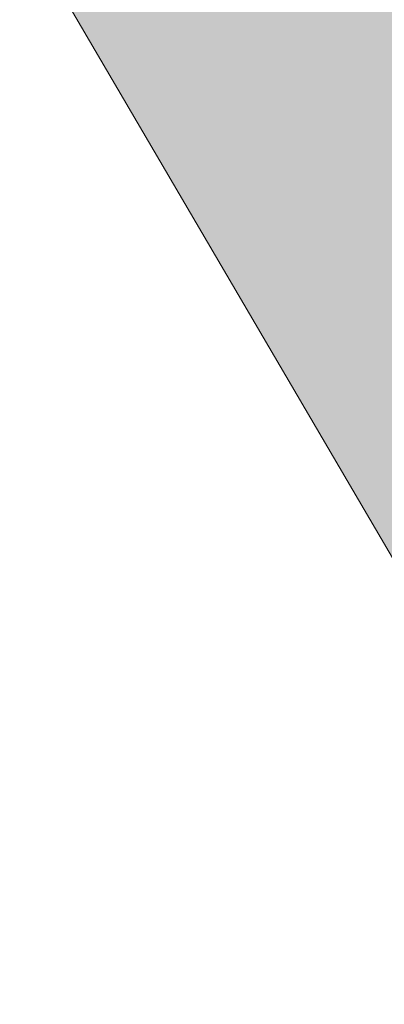
# Model space of a CAD drawing. Units: inches. Extents: x 2091 to 2899, y 967 to 2217.
# Tile 241 of 256: x 2212.556 to 2213.361, y 1133.419 to 1135.592. Entities that reach past the tile are written whole.
import ezdxf

# ---------------------------------------------------------------- set-up
doc = ezdxf.new("R2010")
doc.units = ezdxf.units.IN
doc.layers.add('A-WALL-PATT', color=141, linetype='Continuous', lineweight=13, true_color=0xadddf7)
doc.layers.add('L-PLNT-PATT', color=114, linetype='Continuous', lineweight=13, true_color=0x139b48)
doc.layers.add('L-PLNT-TREE', color=94, linetype='Continuous', lineweight=13)

# ---------------------------------------------------------------- blocks, each defined once
blk = doc.blocks.new('*U25')
blk.add_lwpolyline([(-1139.42368, 1783.79628), (-1216.11644, 1685.47796), (-1117.5111, 1601.2033), (-1051.7759, 1643.3419), (-1126.09884, 1521.20092), (-1072.10606, 1527.49758), (-1079.90386, 1416.93646), (-1259.93906, 1179.83508), (-1479.05978, 1165.78888), (-1577.66258, 1109.60662), (-1742.00312, 927.01364), (-1676.26538, 814.64658), (-1270.89408, 828.69278), (-1194.20386, 772.51052), (-1007.95074, 856.78518), (-876.4778, 575.87134), (-821.70016, 575.87134), (-569.71184, 884.87504)])

msp = doc.modelspace()

# ---------------------------------------------------------------- hatches: boundary and pattern name
at = {"layer": 'A-WALL-PATT'}
h = msp.add_hatch(color=256, dxfattribs=at)
h.dxf.hatch_style = 1
h.paths.add_polyline_path([(2803.1436, 2050.9191), (2203.1436, 2050.9191), (2203.1436, 1090.9191), (2803.1436, 1090.9191)])
h.paths.add_polyline_path([(2635.7989, 1147.5405), (2674.5241, 1147.5405, 0.376086), (2678.5297, 1152.8802), (2678.5297, 1159.5565, 0.333335), (2674.5243, 1163.5618), (2674.5243, 1163.5619), (2674.5243, 1192.9344), (2635.806, 1192.9344), (2597.0876, 1192.9344), (2597.0876, 1163.5618, 0.333335), (2593.0823, 1159.5565), (2593.0823, 1152.8802, 0.376086), (2597.0879, 1147.5405)], flags=0)
h.paths.add_polyline_path([(2436.0104, 1278.2408, 0.000483), (2435.9526, 1278.215, -0.001328), (2435.9356, 1278.1117, -0.001711), (2436.1164, 1278.0408, 0.002185)], flags=0)
h.paths.add_polyline_path([(2794.1436, 1143.4191), (2794.1436, 1347.4191), (2543.3702, 1347.4191), (2543.3702, 1351.9191), (2794.1436, 1351.9191), (2794.1436, 1392.7136), (2793.9474, 1392.7136), (2793.9474, 1473.5369), (2794.1436, 1473.5369), (2794.1436, 1531.9191), (2650.1436, 1531.9191), (2650.1436, 1536.4191), (2794.1436, 1536.4191), (2794.1436, 1692.4191), (2609.3756, 1692.4191), (2609.3756, 1644.4191), (2604.8756, 1644.4191), (2604.8756, 1744.9191), (2609.3756, 1744.9191), (2609.3756, 1696.9191), (2794.1436, 1696.9191), (2794.1436, 1780.9191), (2609.6436, 1780.9191), (2493.8756, 1780.9191), (2493.8756, 1785.4191), (2609.6436, 1785.4191), (2794.1436, 1785.4191), (2794.1436, 1847.9388), (2793.9512, 1847.9388), (2793.9512, 1928.7622), (2794.1436, 1928.7622), (2794.1436, 1941.4191), (2614.1436, 1941.4191), (2614.1436, 1821.4191), (2609.6436, 1821.4191), (2609.6436, 1941.4191), (2392.1436, 1941.4191), (2392.1436, 1819.9191), (2387.6436, 1819.9191), (2387.6436, 1941.4191), (2212.1436, 1941.4191), (2212.1436, 1783.9191), (2392.1436, 1783.9191), (2392.1436, 1780.9191), (2212.1436, 1780.9191), (2212.1436, 1629.4191), (2387.6436, 1629.4191), (2387.6436, 1744.9191), (2392.1436, 1744.9191), (2392.1436, 1627.9191), (2317.1436, 1627.9191), (2317.1436, 1551.4191), (2317.1436, 1536.4191), (2459.3836, 1536.4191), (2459.3836, 1602.3965), (2463.8836, 1602.3965), (2463.8836, 1531.9191), (2456.6436, 1531.9191), (2456.6436, 1529.9191), (2452.1436, 1529.9191), (2452.1436, 1531.9191), (2312.6436, 1531.9191), (2312.6436, 1551.4191), (2306.1436, 1551.4191), (2306.1436, 1555.9191), (2308.1436, 1555.9191), (2308.1436, 1551.4191), (2312.6436, 1551.4191), (2312.6436, 1627.9191), (2212.1436, 1627.9191), (2212.1436, 1555.9191), (2270.1436, 1555.9191), (2270.1436, 1551.4191), (2212.1436, 1551.4191), (2212.1436, 1351.9191), (2272.1436, 1351.9191), (2272.1436, 1347.4191), (2212.1436, 1347.4191), (2212.1436, 1275.4191), (2308.1436, 1275.4191), (2308.1436, 1351.9191), (2452.1436, 1351.9191), (2452.1436, 1493.9191), (2456.6436, 1493.9191), (2456.6436, 1347.4191), (2312.6436, 1347.4191), (2312.6436, 1270.9191), (2212.1436, 1270.9191), (2212.1436, 1099.9191), (2281.2375, 1099.9191), (2282.871, 1110.9138), (2282.0083, 1116.9966), (2278.5577, 1121.4204), (2268.2056, 1128.0562), (2272.0876, 1128.0562), (2273.8129, 1131.927), (2279.4203, 1134.6919), (2285.0278, 1135.2449), (2287.6158, 1137.4568), (2288.0471, 1138.0098), (2289.3411, 1140.7747), (2291.0665, 1139.6687), (2292.3605, 1135.2449), (2295.3798, 1136.9038), (2296.2425, 1135.7979), (2297.1052, 1133.033), (2300.1246, 1138.0098), (2303.1439, 1138.0098), (2304.4379, 1135.7979), (2303.1439, 1133.586), (2306.5946, 1134.6919), (2307.8887, 1133.033), (2310.908, 1135.2449), (2313.9274, 1134.1389), (2315.6269, 1132.4271), (2308.32, 1117.5496), (2290.2038, 1109.8079), (2288.9098, 1103.1721), (2289.2723, 1099.9191), (2434.9182, 1099.9191), (2431.5932, 1124.7881), (2429.9302, 1169.5531), (2430.9272, 1240.5197), (2435.6589, 1238.1861), (2437.1352, 1196.5541), (2438.7982, 1143.9731), (2442.6782, 1111.9981), (2446.5582, 1099.9191), (2794.1436, 1099.9191), (2794.1436, 1138.9191), (2548.0324, 1138.9191), (2548.0324, 1143.4191), (2548.0324, 1148.8191), (2546.6685, 1148.0316), (2528.6857, 1179.1786, 0.256256), (2512.0324, 1148.8191), (2512.0324, 1143.4191), (2512.0324, 1138.9191), (2507.5324, 1138.9191), (2507.5324, 1143.4191), (2507.5324, 1148.8191, 0.256256), (2490.8792, 1179.1786), (2472.8964, 1148.0316), (2471.5324, 1148.8191), (2471.5324, 1143.4191), (2467.0324, 1143.4191), (2467.0324, 1269.9458, 0.039061), (2460.91, 1273.5801), (2467.0324, 1273.5801), (2467.0324, 1286.3254, 0.014511), (2465.2162, 1286.7619), (2467.0324, 1287.0526), (2467.0324, 1323.4191), (2471.5324, 1323.4191), (2471.5324, 1148.8191), (2489.5324, 1179.996), (2490.8964, 1179.2085), (2490.8792, 1179.1786, -0.256256), (2507.5324, 1148.8191), (2507.5324, 1143.4191), (2512.0324, 1143.4191), (2512.0324, 1148.8191, -0.256256), (2528.6857, 1179.1786), (2528.6685, 1179.2085), (2530.0324, 1179.996), (2548.0324, 1148.8191), (2548.0324, 1143.4191)], flags=16)
h.paths.add_polyline_path([(2607.7685, 1200.9451), (2607.7685, 1265.0306), (2597.0876, 1281.052), (2619.7846, 1281.052), (2627.7953, 1337.1269), (2635.7989, 1337.1269), (2643.8167, 1337.1269), (2651.8274, 1281.052), (2674.5243, 1281.052), (2663.8434, 1265.0306), (2663.8434, 1200.9451), (2635.806, 1200.9451)], flags=0)
edge = h.paths.add_edge_path(flags=0)
edge.add_ellipse((13303.8962, 1272.9987), major_axis=(-10595.313, 0), ratio=0.8423038701, start_angle=0.62823722, end_angle=0.6465541, ccw=False)
edge.add_ellipse((2711.7004, 1156.8527), major_axis=(2.2198, 0), ratio=0.842304, start_angle=111.5352, end_angle=180.6282, ccw=False)
edge.add_ellipse((13303.1563, 1272.9987), major_axis=(-10593.0263, 0), ratio=0.8423038695, start_angle=0.52827147, end_angle=0.6465541, ccw=False)
edge.add_line((2710.7646, 1175.3333), (2710.13, 1175.3333))
edge.add_ellipse((2710.13, 1176.5798), major_axis=(1.4798, 0), ratio=0.842304, start_angle=180, end_angle=270, ccw=False)
edge.add_line((2708.6501, 1176.5798), (2708.6501, 1200.7829))
edge.add_ellipse((2710.13, 1200.7829), major_axis=(1.4798, 0), ratio=0.842304, start_angle=90, end_angle=180, ccw=False)
edge.add_line((2710.13, 1202.0294), (2710.4651, 1202.0294))
edge.add_ellipse((13303.1563, 1272.9987), major_axis=(-10593.0263, 0), ratio=0.8423038695, start_angle=-0.09022909, end_angle=0.38386678, ccw=False)
edge.add_ellipse((2710.13, 1290.927), major_axis=(-1.4798, 0), ratio=0.842304, start_angle=0, end_angle=90, ccw=False)
edge.add_line((2708.6501, 1290.927), (2708.6501, 1315.1302))
edge.add_ellipse((2710.13, 1315.1302), major_axis=(-1.4798, 0), ratio=0.842304, start_angle=-90, end_angle=0, ccw=False)
edge.add_line((2710.13, 1316.3767), (2710.7063, 1316.3767))
edge.add_ellipse((3238.4017, 1296.2896), major_axis=(528.234, 0), ratio=0.84230387, start_angle=176.349572, end_angle=177.82005, ccw=False)
edge.add_ellipse((2775.063, 1071.4507), major_axis=(313.3078, 0), ratio=0.84230387, start_angle=102.125966, end_angle=103.780529, ccw=False)
edge.add_ellipse((2775.063, 1078.3057), major_axis=(-305.3029, 0), ratio=0.84230387, start_angle=-79.790461, end_angle=-77.555373, ccw=False)
edge.add_ellipse((2695.1418, 1541.9754), major_axis=(-250.9602, 0), ratio=0.84230387, start_angle=99.256566, end_angle=102.554933)
edge.add_line((2741.4103, 1334.2143), (2747.1325, 1337.3785))
edge.add_ellipse((2747.5386, 1336.8575), major_axis=(-0.7399, 0), ratio=0.842304, start_angle=270, end_angle=307.9331, ccw=False)
edge.add_ellipse((2747.5386, 1336.8575), major_axis=(-0.7399, 0), ratio=0.842304, start_angle=232.0669, end_angle=270, ccw=False)
edge.add_line((2747.9447, 1337.3785), (2753.6669, 1334.2143))
edge.add_ellipse((2799.9355, 1541.9754), major_axis=(250.9602, 0), ratio=0.84230387, start_angle=257.445067, end_angle=260.743434)
edge.add_ellipse((2720.0142, 1078.3057), major_axis=(305.3029, 0), ratio=0.84230387, start_angle=77.555373, end_angle=79.790461, ccw=False)
edge.add_ellipse((2720.0142, 1071.4507), major_axis=(-313.3078, 0), ratio=0.84230387, start_angle=256.219471, end_angle=257.874034, ccw=False)
edge.add_ellipse((2256.6755, 1296.2896), major_axis=(-528.234, 0), ratio=0.84230387, start_angle=182.17995, end_angle=183.650428, ccw=False)
edge.add_line((2784.3709, 1316.3767), (2784.9472, 1316.3767))
edge.add_ellipse((2784.9472, 1315.1302), major_axis=(1.4798, 0), ratio=0.842304, start_angle=0, end_angle=90, ccw=False)
edge.add_line((2786.4271, 1315.1302), (2786.4271, 1290.927))
edge.add_ellipse((2784.9472, 1290.927), major_axis=(1.4798, 0), ratio=0.842304, start_angle=270, end_angle=360, ccw=False)
edge.add_ellipse((-7808.0791, 1272.9987), major_axis=(10593.0263, 0), ratio=0.8423038695, start_angle=-0.38386678, end_angle=0.09022909, ccw=False)
edge.add_line((2784.6122, 1202.0294), (2784.9472, 1202.0294))
edge.add_ellipse((2784.9472, 1200.7829), major_axis=(1.4798, 0), ratio=0.842304, start_angle=0, end_angle=90, ccw=False)
edge.add_line((2786.4271, 1200.7829), (2786.4271, 1176.5798))
edge.add_ellipse((2784.9472, 1176.5798), major_axis=(-1.4798, 0), ratio=0.842304, start_angle=90, end_angle=180, ccw=False)
edge.add_line((2784.9472, 1175.3333), (2784.3126, 1175.3333))
edge.add_ellipse((-7808.0791, 1272.9987), major_axis=(10593.0263, 0), ratio=0.8423038695, start_angle=-0.6186432, end_angle=-0.52827147, ccw=False)
edge.add_ellipse((2783.3768, 1156.8527), major_axis=(-2.2198, 0), ratio=0.842304, start_angle=179.3718, end_angle=248.4648, ccw=False)
edge.add_ellipse((-7808.819, 1272.9987), major_axis=(-10595.313, 0), ratio=0.8423038658, start_angle=179.35344592, end_angle=179.3717628, ccw=False)
edge.add_ellipse((2780.2973, 1153.5008), major_axis=(-5.2464, 0), ratio=0.842304, start_angle=90, end_angle=179.3534, ccw=False)
edge.add_line((2780.2973, 1149.0817), (2714.7799, 1149.0817))
edge.add_ellipse((2714.7799, 1153.5008), major_axis=(5.2464, 0), ratio=0.842304, start_angle=180.6466, end_angle=270, ccw=False)
edge = h.paths.add_edge_path(flags=0)
edge.add_line((2718.1874, 1151.0078), (2718.1874, 1170.4724))
edge.add_ellipse((2721.1471, 1170.4724), major_axis=(-2.9597, 0), ratio=0.842304, start_angle=-90, end_angle=0, ccw=False)
edge.add_line((2721.1471, 1172.9653), (2773.9302, 1172.9653))
edge.add_ellipse((2773.9302, 1170.4724), major_axis=(-2.9597, 0), ratio=0.842304, start_angle=180, end_angle=270, ccw=False)
edge.add_line((2776.8899, 1170.4724), (2776.8899, 1151.0078))
edge.add_line((2776.8899, 1151.0078), (2718.1874, 1151.0078))
edge = h.paths.add_edge_path(flags=0)
edge.add_line((2718.1874, 1180.2342), (2718.1874, 1199.0578))
edge.add_ellipse((2747.5386, 1320.3986), major_axis=(147.0179, 0), ratio=0.84230387, start_angle=256.401865, end_angle=283.598135)
edge.add_line((2776.8899, 1199.0578), (2776.8899, 1180.2342))
edge.add_ellipse((2747.5386, 1301.575), major_axis=(147.0179, 0), ratio=0.84230387, start_angle=256.401865, end_angle=283.598135, ccw=False)
edge = h.paths.add_edge_path(flags=0)
edge.add_ellipse((13303.1563, 1272.9987), major_axis=(-10591.5465, 0), ratio=0.8423038696, start_angle=0.05559431, end_angle=0.37776419, ccw=False)
edge.add_line((2711.6169, 1262.7217), (2715.6674, 1249.4954))
edge.add_ellipse((6413.892, 1241.6919), major_axis=(-3698.2362, 0), ratio=0.84230387, start_angle=-0.1208974, end_angle=0.3640763)
edge.add_line((2715.761, 1218.1925), (2711.9343, 1203.1674))
edge = h.paths.add_edge_path(flags=0)
edge.add_line((2718.1874, 1251.0746), (2716.0025, 1267.4504))
edge.add_ellipse((2742.1512, 1202.1895), major_axis=(81.7726, 0), ratio=0.8423039, start_angle=94.277421, end_angle=111.834954, ccw=False)
edge.add_line((2737.0097, 1270.9306), (2758.0675, 1270.9306))
edge.add_ellipse((2752.9261, 1202.1895), major_axis=(81.7726, 0), ratio=0.8423039, start_angle=68.165046, end_angle=85.722579, ccw=False)
edge.add_line((2779.0747, 1267.4504), (2776.8899, 1251.0746))
edge.add_ellipse((2750.3381, 1187.8854), major_axis=(79.5797, 0), ratio=0.8423039, start_angle=67.208085, end_angle=85.12993)
edge.add_line((2756.0347, 1254.7437), (2739.0426, 1254.7437))
edge.add_ellipse((2744.7392, 1187.8854), major_axis=(79.5797, 0), ratio=0.8423039, start_angle=94.87007, end_angle=112.791915)
edge = h.paths.add_edge_path(flags=0)
edge.add_line((2783.1429, 1203.1674), (2779.3162, 1218.1925))
edge.add_ellipse((-918.8147, 1241.6919), major_axis=(3698.2362, 0), ratio=0.84230387, start_angle=-0.3640763, end_angle=0.1208974)
edge.add_line((2779.4098, 1249.4954), (2783.4604, 1262.7217))
edge.add_ellipse((-7808.0791, 1272.9987), major_axis=(-10591.5465, 0), ratio=0.8423038695, start_angle=179.62223581, end_angle=179.94440569, ccw=False)
edge = h.paths.add_edge_path(flags=0)
edge.add_ellipse((2734.2009, 1286.6904), major_axis=(-0.3566, 6.3401), ratio=0.603834, start_angle=89.00201, end_angle=253.65741, ccw=False)
edge.add_line((2730.369, 1286.5418), (2730.369, 1301.352))
edge.add_line((2730.369, 1301.352), (2735.9133, 1305.2148))
edge.add_ellipse((2736.3849, 1304.7346), major_axis=(0.7399, 0), ratio=0.842304, start_angle=90, end_angle=134.4802, ccw=False)
edge.add_line((2736.3849, 1305.3578), (2738.0328, 1305.3578))
edge.add_line((2738.0328, 1305.3578), (2738.0328, 1307.7079))
edge.add_ellipse((2794.2016, 1307.7079), major_axis=(56.1689, 0), ratio=0.8423039, start_angle=150.56143, end_angle=180, ccw=False)
edge.add_ellipse((2700.8756, 1307.7079), major_axis=(-56.1689, 0), ratio=0.8423039, start_angle=180, end_angle=209.43857, ccw=False)
edge.add_line((2757.0444, 1307.7079), (2757.0444, 1305.3578))
edge.add_line((2757.0444, 1305.3578), (2758.6923, 1305.3578))
edge.add_ellipse((2758.6923, 1304.7346), major_axis=(-0.7399, 0), ratio=0.842304, start_angle=225.5198, end_angle=270, ccw=False)
edge.add_line((2759.1639, 1305.2148), (2764.7082, 1301.352))
edge.add_line((2764.7082, 1301.352), (2764.7082, 1286.5418))
edge.add_ellipse((2760.8763, 1286.6904), major_axis=(0.3566, 6.3401), ratio=0.603834, start_angle=106.34259, end_angle=270.99799, ccw=False)
edge.add_line((2757.0444, 1285.7971), (2757.0444, 1307.7079))
edge.add_ellipse((2700.8756, 1307.7079), major_axis=(-56.1689, 0), ratio=0.8423039, start_angle=180, end_angle=209.43857)
edge.add_ellipse((2794.2016, 1307.7079), major_axis=(56.1689, 0), ratio=0.8423039, start_angle=150.56143, end_angle=180)
edge.add_line((2738.0328, 1307.7079), (2738.0328, 1285.7971))
h.paths.add_polyline_path([(2417.8123, 1104.4497), (2413.4923, 1102.5297), (2410.6123, 1103.9697), (2409.1723, 1106.3697), (2407.2523, 1107.3297), (2406.2923, 1109.7297), (2405.3323, 1114.0497), (2405.3323, 1117.8897), (2406.2923, 1120.1297), (2407.2523, 1119.8097), (2408.8483, 1118.3277), (2410.1739, 1119.4242), (2410.2113, 1120.4057), (2411.0407, 1121.4191), (2410.6993, 1119.8587), (2410.1739, 1119.4242), (2410.0885, 1117.1761), (2411.1328, 1116.2063), (2413.9723, 1119.3297), (2416.8523, 1120.7697), (2416.8697, 1120.7988), (2417.0351, 1119.4051), (2417.8962, 1118.1434), (2418.2923, 1118.3697), (2419.5444, 1120.0393), (2419.3609, 1118.3875), (2419.0321, 1119.3562), (2418.3989, 1118.5119), (2419.2523, 1114.5297), (2418.7941, 1107.1988)], flags=0)
h.paths.add_polyline_path([(2508.8702, 1347.4191), (2508.3702, 1347.4191), (2508.3702, 1351.9191), (2508.8702, 1351.9191)], flags=0)
h.paths.add_polyline_path([(2473.3702, 1347.4191), (2472.3702, 1347.4191), (2467.8702, 1347.4191), (2467.8702, 1455.4191), (2472.3702, 1455.4191), (2472.3702, 1352.4191), (2473.3702, 1352.4191)], flags=0)
h.paths.add_polyline_path([(2352.1062, 1217.4462), (2349.2262, 1218.8862), (2347.7862, 1221.2862), (2345.8662, 1222.2462), (2344.9062, 1224.6462), (2343.9462, 1228.9662), (2343.9462, 1232.8062), (2344.9062, 1235.0462), (2345.8662, 1234.7262), (2347.4623, 1233.2442), (2348.7879, 1234.3407), (2348.8252, 1235.3222), (2349.6547, 1236.3355), (2349.3132, 1234.7752), (2348.7879, 1234.3407), (2348.7024, 1232.0926), (2349.7468, 1231.1228), (2352.5862, 1234.2462), (2355.4662, 1235.6862), (2355.4837, 1235.7153), (2355.649, 1234.3216), (2356.5102, 1233.0599), (2356.9062, 1233.2862), (2358.1584, 1234.9558), (2357.9749, 1233.304), (2357.6461, 1234.2726), (2357.0129, 1233.4284), (2357.8662, 1229.4462), (2357.4081, 1222.1153), (2356.4262, 1219.3662)], flags=0)
h.paths.add_polyline_path([(2348.2968, 1112.2244), (2347.0138, 1112.3104), (2345.5298, 1114.1274), (2345.7318, 1115.8584), (2346.8118, 1116.9824), (2346.8118, 1114.6464), (2345.8668, 1114.2144), (2346.8798, 1114.3004)], flags=0)
h.paths.add_polyline_path([(2347.0138, 1110.9264), (2346.2718, 1110.4934), (2346.6098, 1111.1864)], flags=0)
h.paths.add_polyline_path([(2345.8668, 1118.1944), (2345.5298, 1117.3294), (2343.7078, 1118.0214), (2344.3828, 1118.6264)], flags=0)
h.paths.add_polyline_path([(2346.6768, 1109.2824), (2346.0698, 1108.0714), (2345.8668, 1110.0614)], flags=0)
h.paths.add_polyline_path([(2345.0568, 1119.7514), (2343.6398, 1119.7514), (2343.9778, 1121.1354)], flags=0)
h.paths.add_polyline_path([(2345.2598, 1116.5504), (2345.1248, 1115.8584), (2344.9218, 1115.6854), (2344.7198, 1116.3774)], flags=0)
h.paths.add_polyline_path([(2345.6648, 1112.3104), (2345.4618, 1111.5324), (2344.0448, 1111.9644), (2344.6518, 1112.5704)], flags=0)
h.paths.add_polyline_path([(2345.1918, 1113.3494), (2344.4498, 1113.8684), (2344.7198, 1114.3874)], flags=0)
h.paths.add_polyline_path([(2344.6518, 1116.8094), (2344.1798, 1115.6854), (2344.6518, 1115.3394), (2343.9098, 1114.9064), (2343.0328, 1115.9444), (2343.6398, 1116.4634)], flags=0)
h.paths.add_polyline_path([(2345.8668, 1106.6864), (2344.9898, 1105.5624), (2344.5168, 1106.6004)], flags=0)
h.paths.add_polyline_path([(2344.8548, 1110.0614), (2344.5168, 1109.2824), (2344.1128, 1109.7154)], flags=0)
h.paths.add_polyline_path([(2344.0448, 1113.5224), (2343.4378, 1113.0894), (2342.7628, 1113.9544)], flags=0)
h.paths.add_polyline_path([(2344.3148, 1111.0124), (2342.9648, 1110.3204), (2342.9648, 1111.0994)], flags=0)
h.paths.add_polyline_path([(2345.1248, 1104.6974), (2344.5848, 1103.7454), (2344.4498, 1104.2644)], flags=0)
h.paths.add_polyline_path([(2342.8298, 1121.2224), (2341.7498, 1120.5304), (2340.5358, 1121.0494), (2340.1308, 1121.8284), (2340.6708, 1122.9524), (2341.1428, 1121.8284), (2341.6148, 1122.0014)], flags=0)
h.paths.add_polyline_path([(2342.9648, 1119.7514), (2343.0328, 1118.4534), (2342.0878, 1118.0214), (2342.0198, 1119.4914)], flags=0)
h.paths.add_polyline_path([(2342.6948, 1116.8964), (2341.9528, 1116.6364), (2342.0198, 1117.3294)], flags=0)
h.paths.add_polyline_path([(2343.0328, 1112.2244), (2342.0198, 1111.7914), (2341.5478, 1112.2244), (2342.3578, 1113.3494)], flags=0)
h.paths.add_polyline_path([(2343.7748, 1104.4374), (2342.6278, 1102.8804), (2342.6948, 1104.6104), (2343.4378, 1105.1294)], flags=0)
h.paths.add_polyline_path([(2342.0198, 1115.0794), (2340.8058, 1115.5124), (2340.9408, 1116.3774)], flags=0)
h.paths.add_polyline_path([(2341.4808, 1120.0974), (2341.4808, 1119.4054), (2341.0758, 1119.5784), (2341.1428, 1120.0974)], flags=0)
h.paths.add_polyline_path([(2341.8178, 1114.4734), (2340.9408, 1113.0894), (2340.8058, 1114.5604)], flags=0)
h.paths.add_polyline_path([(2341.1428, 1118.5404), (2340.9408, 1116.9824), (2339.0508, 1117.6754), (2339.0508, 1118.6264)], flags=0)
h.paths.add_polyline_path([(2342.6948, 1101.6684), (2341.9528, 1101.8414), (2342.5598, 1102.3614)], flags=0)
h.paths.add_polyline_path([(2340.3328, 1119.6654), (2338.4438, 1119.5784), (2337.9038, 1120.3574), (2339.6578, 1120.6164)], flags=0)
h.paths.add_polyline_path([(2340.3328, 1115.3394), (2340.0628, 1113.6954), (2339.3878, 1115.3394)], flags=0)
h.paths.add_polyline_path([(2341.8178, 1103.8314), (2341.5478, 1102.8804), (2341.1428, 1103.6584)], flags=0)
h.paths.add_polyline_path([(2339.0508, 1122.8664), (2337.2958, 1121.8284), (2337.0938, 1123.1254), (2337.7688, 1123.8184)], flags=0)
h.paths.add_polyline_path([(2339.1178, 1121.7414), (2338.8478, 1121.2224), (2338.1738, 1121.0494), (2338.3758, 1121.5684)], flags=0)
h.paths.add_polyline_path([(2339.1858, 1119.3194), (2338.6458, 1118.7134), (2338.2408, 1118.1074), (2338.2408, 1118.8864)], flags=0)
h.paths.add_polyline_path([(2341.1428, 1101.9284), (2340.6028, 1101.2364), (2340.0628, 1101.8414), (2340.6028, 1102.3614)], flags=0)
h.paths.add_polyline_path([(2337.6338, 1117.7614), (2336.6208, 1118.2804), (2337.2958, 1118.9724)], flags=0)
h.paths.add_polyline_path([(2336.8238, 1119.5784), (2334.7988, 1118.9724), (2335.2038, 1120.3574), (2336.5538, 1120.8764)], flags=0)
h.paths.add_polyline_path([(2339.1178, 1100.4574), (2337.3638, 1100.5434), (2336.7558, 1101.2364)], flags=0)
h.paths.add_polyline_path([(2336.3508, 1122.4334), (2336.0138, 1121.9144), (2334.9338, 1122.4334), (2334.5288, 1123.4714), (2335.7438, 1122.7794)], flags=0)
h.paths.add_polyline_path([(2334.7318, 1120.8764), (2334.2588, 1120.3574), (2334.0568, 1120.7894), (2334.5968, 1121.3084)], flags=0)
h.paths.add_polyline_path([(2334.4618, 1122.1744), (2332.5718, 1121.3084), (2331.3568, 1122.1744), (2332.0998, 1122.8664)], flags=0)
h.paths.add_polyline_path([(2334.2588, 1118.5404), (2333.3818, 1118.4534), (2333.6518, 1119.3194)], flags=0)
h.paths.add_polyline_path([(2335.5418, 1102.2744), (2334.1918, 1102.6204), (2335.2718, 1103.3124)], flags=0)
h.paths.add_polyline_path([(2332.7068, 1119.6654), (2331.6948, 1120.4434), (2332.5048, 1120.7894)], flags=0)
h.paths.add_polyline_path([(2334.7318, 1101.1494), (2333.5168, 1101.5824), (2333.9888, 1101.7554)], flags=0)
h.paths.add_polyline_path([(2332.6398, 1116.6364), (2331.0868, 1116.2904), (2331.9648, 1118.1944)], flags=0)
h.paths.add_polyline_path([(2330.7498, 1121.5684), (2330.2768, 1120.2704), (2328.5228, 1119.3194), (2328.9948, 1121.0494)], flags=0)
h.paths.add_polyline_path([(2330.7498, 1118.6264), (2330.0078, 1117.5024), (2329.8728, 1118.0214)], flags=0)
h.paths.add_polyline_path([(2332.0998, 1102.3614), (2330.5468, 1102.0144), (2331.6948, 1102.9664)], flags=0)
h.paths.add_polyline_path([(2329.5348, 1113.6084), (2329.0628, 1112.3104), (2328.5898, 1113.3494)], flags=0)
h.paths.add_polyline_path([(2328.3878, 1117.8484), (2327.5098, 1116.5504), (2327.1728, 1117.7614)], flags=0)
h.paths.add_polyline_path([(2329.7378, 1106.5134), (2329.5348, 1105.3024), (2328.2528, 1106.0814)], flags=0)
h.paths.add_polyline_path([(2328.6578, 1114.3874), (2328.0498, 1114.1274), (2328.3198, 1114.9064)], flags=0)
h.paths.add_polyline_path([(2328.3198, 1112.2244), (2327.1058, 1112.1374), (2326.7008, 1112.6564)], flags=0)
h.paths.add_polyline_path([(2326.9028, 1115.2524), (2326.7008, 1114.1274), (2325.2158, 1113.6084), (2326.0928, 1115.3394)], flags=0)
h.paths.add_polyline_path([(2326.6328, 1108.3304), (2326.0928, 1107.3794), (2325.8908, 1108.5034), (2326.4978, 1109.1094)], flags=0)
h.paths.add_polyline_path([(2615.1436, 1531.9191), (2609.6436, 1531.9191), (2609.6436, 1620.4191), (2614.1436, 1620.4191), (2614.1436, 1536.4191), (2615.1436, 1536.4191)], flags=0)
h.paths.add_polyline_path([(2545.1436, 1563.4191), (2464.1436, 1563.4191), (2464.1436, 1632.4191), (2509.1436, 1632.4191), (2509.1436, 1627.9191), (2509.1436, 1603.9191), (2468.6436, 1603.9191), (2468.6436, 1567.9191), (2540.6436, 1567.9191), (2540.6436, 1591.9191), (2545.1436, 1591.9191)], flags=0)
h.paths.add_polyline_path([(2388.969, 1549.9857), (2357.4342, 1549.9857), (2357.4342, 1623.3608), (2399.3628, 1623.3608), (2435.6895, 1623.3608), (2435.5925, 1602.5593), (2435.5925, 1602.3965), (2388.969, 1602.3965)], flags=0)
h.paths.add_polyline_path([(2388.8806, 1555.8092), (2374.9044, 1555.8092), (2374.9044, 1600.5716), (2374.9044, 1615.4576), (2406.3509, 1615.4576), (2406.3509, 1618.9394), (2412.1743, 1615.4576), (2406.3509, 1611.9759), (2406.3509, 1615.4576), (2388.8806, 1615.4576)], flags=0)
h.paths.add_polyline_path([(2568.8756, 1644.4191), (2453.3756, 1644.4191), (2453.3756, 1785.4191), (2457.8756, 1785.4191), (2457.8756, 1648.9191), (2568.8756, 1648.9191)], flags=0)
h.paths.add_polyline_path([(2212.1436, 1945.9191), (2212.1436, 2041.9191), (2794.1436, 2041.9191), (2794.1436, 1945.9191)], flags=16)
h.paths.add_polyline_path([(2271.0827, 1964.3172), (2776.853, 1964.3172), (2776.853, 2037.1696), (2271.0827, 2037.1696)], flags=8)
h.paths.add_polyline_path([(2380.6493, 1536.8241), (2461.0408, 1536.8241), (2461.0408, 1554.6526), (2380.6493, 1554.6526)], flags=8)
h.paths.add_polyline_path([(2240.7557, 1609.7255), (2309.1858, 1609.7255), (2309.1858, 1617.6982), (2240.7557, 1617.6982)], flags=8)
h.paths.add_polyline_path([(2212.6773, 1313.5041), (2282.5915, 1313.5041), (2282.5915, 1322.7452), (2212.6773, 1322.7452)], flags=8)
h.paths.add_polyline_path([(2457.112, 1114.7786), (2558.4816, 1114.7786), (2558.4816, 1142.2197), (2457.112, 1142.2197)], flags=8)
h.paths.add_polyline_path([(2473.4423, 1273.0101), (2604.6412, 1273.0101), (2604.6412, 1318.3469), (2473.4423, 1318.3469)], flags=8)
h.paths.add_polyline_path([(2638.8763, 1626.9774), (2684.2504, 1627.9767), (2684.0385, 1637.5975), (2638.6644, 1636.5982)], flags=8)
h.paths.add_polyline_path([(2537.5906, 1453.7934), (2628.3895, 1453.7934), (2628.3895, 1475.3448), (2537.5906, 1475.3448)], flags=8)
h.paths.add_polyline_path([(2504.1376, 1714.6324), (2554.6472, 1714.6324), (2554.6472, 1730.2377), (2504.1376, 1730.2377)], flags=8)
h.paths.add_polyline_path([(2487.5012, 1575.6519), (2535.0971, 1575.6519), (2535.0971, 1598.3776), (2487.5012, 1598.3776)], flags=8)
h.paths.add_polyline_path([(2709.0994, 1735.7103), (2740.0166, 1735.7103), (2740.0166, 1749.9376), (2709.0994, 1749.9376)], flags=8)
h.paths.add_polyline_path([(2442.4384, 1792.1717), (2564.7288, 1792.1717), (2564.7288, 1842.0002), (2442.4384, 1842.0002)], flags=8)
h.paths.add_polyline_path([(2655.8158, 1809.6441), (2789.5201, 1806.6938), (2790.085, 1832.2916), (2656.3806, 1835.2419)], flags=8)
h.paths.add_polyline_path([(2234.8427, 1797.7201), (2368.5929, 1794.7689), (2369.1607, 1820.5041), (2235.4106, 1823.4554)], flags=8)
h.paths.add_polyline_path([(2245.1385, 1644.0063), (2398.4277, 1640.6239), (2398.9948, 1666.3248), (2245.7056, 1669.7073)], flags=8)
h.paths.add_polyline_path([(2306.1428, 1431.1685), (2413.7683, 1428.7937), (2414.3331, 1454.3915), (2306.7077, 1456.7664)], flags=8)
h.paths.add_polyline_path([(2306.8346, 1458.2331), (2393.3805, 1456.3234), (2393.9328, 1481.3544), (2307.3869, 1483.2641)], flags=8)
at = {"layer": 'L-PLNT-PATT'}
h = msp.add_hatch(color=256, dxfattribs=at)
h.dxf.hatch_style = 1
h.paths.add_polyline_path([(2333.3376, 1165.6587), (2329.0242, 1166.2116), (2331.6122, 1168.4235), (2335.0629, 1177.2712), (2328.1615, 1184.4599), (2319.5348, 1187.2248), (2323.4168, 1193.3076), (2319.9661, 1203.8142), (2317.8094, 1203.8142), (2313.496, 1213.2148), (2310.908, 1212.6618), (2307.8887, 1212.6618), (2305.7319, 1217.0857), (2307.0259, 1223.1684), (2310.4767, 1223.1684), (2304.0066, 1230.9101), (2303.1363, 1237.0465), (2299.6932, 1240.8637), (2296.6739, 1237.5459), (2294.9485, 1238.6518), (2294.5171, 1241.4166), (2292.3605, 1242.5227), (2289.3411, 1239.7577), (2285.8904, 1240.3107), (2283.3024, 1235.3339), (2283.3024, 1230.9101), (2286.7531, 1229.2512), (2284.165, 1227.5922), (2281.577, 1229.8042), (2274.2442, 1222.6154), (2274.2442, 1220.9565), (2271.2249, 1219.2976), (2272.0876, 1217.6386), (2274.2442, 1214.3208), (2270.3622, 1211.5559), (2266.4801, 1214.3208), (2264.3235, 1213.7678), (2263.4608, 1211.5559), (2266.4801, 1211.0029), (2266.9115, 1206.5791), (2263.5392, 1207.132), (2259.5788, 1203.2612), (2263.8921, 1202.7082), (2262.1668, 1197.1784), (2258.2848, 1196.6254), (2253.9714, 1193.8606), (2248.7953, 1191.0957), (2248.364, 1193.3076), (2244.4819, 1185.0129), (2251.3833, 1186.6718), (2255.6967, 1183.9069), (2254.4027, 1177.2712), (2246.6387, 1174.5063), (2243.1879, 1176.7182), (2241.8939, 1173.4003), (2238.8746, 1172.8474), (2236.2865, 1169.5295), (2233.2671, 1165.6587), (2237.1492, 1162.3408), (2239.7372, 1163.9998), (2236.8111, 1159.1911), (2238.9368, 1159.439), (2238.6298, 1155.0862), (2231.5418, 1145.7515), (2222.915, 1145.1985), (2219.033, 1142.9866), (2212.5629, 1135.7979), (2215.151, 1131.374), (2231.1105, 1131.927), (2234.1298, 1129.7151), (2241.4626, 1133.033), (2246.6387, 1121.9734), (2248.7953, 1121.9734), (2258.7161, 1134.1389), (2261.7355, 1135.7979), (2263.8921, 1133.033), (2263.8921, 1129.1621), (2267.3429, 1128.0562), (2272.0876, 1128.0562), (2273.8129, 1131.927), (2279.4203, 1134.6919), (2285.0278, 1135.2449), (2287.6158, 1137.4568), (2288.0471, 1138.0098), (2289.3411, 1140.7747), (2291.0665, 1139.6687), (2292.3605, 1135.2449), (2295.3798, 1136.9038), (2296.2425, 1135.7979), (2297.1052, 1133.033), (2300.1246, 1138.0098), (2303.1439, 1138.0098), (2304.4379, 1135.7979), (2303.1439, 1133.586), (2306.5946, 1134.6919), (2307.8887, 1133.033), (2310.908, 1135.2449), (2313.9274, 1134.1389), (2319.9661, 1128.0562), (2322.5541, 1126.9502), (2324.7108, 1124.7383), (2342.827, 1126.3972), (2346.2777, 1123.0794), (2348.8658, 1124.1853), (2341.9643, 1133.033), (2341.533, 1136.3508), (2343.6897, 1139.6687), (2339.8077, 1150.1753), (2337.651, 1150.1753)])
h.paths.add_polyline_path([(2339.6578, 1120.6164), (2337.9038, 1120.3574), (2338.4438, 1119.5784), (2340.3328, 1119.6654)])
h.paths.add_polyline_path([(2341.1428, 1118.5404), (2339.0508, 1118.6264), (2339.0508, 1117.6754), (2340.9408, 1116.9824)])
h.paths.add_polyline_path([(2336.5538, 1120.8764), (2335.2038, 1120.3574), (2334.7988, 1118.9724), (2336.8238, 1119.5784)])
h.paths.add_polyline_path([(2337.2958, 1118.9724), (2336.6208, 1118.2804), (2337.6338, 1117.7614)])
h.paths.add_polyline_path([(2338.6458, 1118.7134), (2339.1858, 1119.3194), (2338.2408, 1118.8864), (2338.2408, 1118.1074)])
h.paths.add_polyline_path([(2339.0508, 1122.8664), (2337.7688, 1123.8184), (2337.0938, 1123.1254), (2337.2958, 1121.8284)])
h.paths.add_polyline_path([(2341.6148, 1122.0014), (2341.1428, 1121.8284), (2340.6708, 1122.9524), (2340.1308, 1121.8284), (2340.5358, 1121.0494), (2341.7498, 1120.5304), (2342.8298, 1121.2224)])
h.paths.add_polyline_path([(2342.9648, 1119.7514), (2342.0198, 1119.4914), (2342.0878, 1118.0214), (2343.0328, 1118.4534)])
h.paths.add_polyline_path([(2345.8668, 1118.1944), (2344.3828, 1118.6264), (2343.7078, 1118.0214), (2345.5298, 1117.3294)])
h.paths.add_polyline_path([(2344.6518, 1116.8094), (2343.6398, 1116.4634), (2343.0328, 1115.9444), (2343.9098, 1114.9064), (2344.6518, 1115.3394), (2344.1798, 1115.6854)])
h.paths.add_polyline_path([(2346.8118, 1116.9824), (2345.7318, 1115.8584), (2345.5298, 1114.1274), (2347.0138, 1112.3104), (2348.2968, 1112.2244), (2346.8798, 1114.3004), (2345.8668, 1114.2144), (2346.8118, 1114.6464)])
h.paths.add_polyline_path([(2345.2598, 1116.5504), (2344.7198, 1116.3774), (2344.9218, 1115.6854), (2345.1248, 1115.8584)])
h.paths.add_polyline_path([(2342.6948, 1116.8964), (2342.0198, 1117.3294), (2341.9528, 1116.6364)])
h.paths.add_polyline_path([(2341.4808, 1120.0974), (2341.1428, 1120.0974), (2341.0758, 1119.5784), (2341.4808, 1119.4054)])
h.paths.add_polyline_path([(2343.9778, 1121.1354), (2343.6398, 1119.7514), (2345.0568, 1119.7514)])
h.paths.add_polyline_path([(2339.1178, 1121.7414), (2338.3758, 1121.5684), (2338.1738, 1121.0494), (2338.8478, 1121.2224)])
h.paths.add_polyline_path([(2336.3508, 1122.4334), (2335.7438, 1122.7794), (2334.5288, 1123.4714), (2334.9338, 1122.4334), (2336.0138, 1121.9144)])
h.paths.add_polyline_path([(2334.4618, 1122.1744), (2332.0998, 1122.8664), (2331.3568, 1122.1744), (2332.5718, 1121.3084)])
h.paths.add_polyline_path([(2334.5968, 1121.3084), (2334.0568, 1120.7894), (2334.2588, 1120.3574), (2334.7318, 1120.8764)])
h.paths.add_polyline_path([(2332.5048, 1120.7894), (2331.6948, 1120.4434), (2332.7068, 1119.6654)])
h.paths.add_polyline_path([(2333.6518, 1119.3194), (2333.3818, 1118.4534), (2334.2588, 1118.5404)])
h.paths.add_polyline_path([(2331.9648, 1118.1944), (2331.0868, 1116.2904), (2332.6398, 1116.6364)])
h.paths.add_polyline_path([(2330.7498, 1121.5684), (2328.9948, 1121.0494), (2328.5228, 1119.3194), (2330.2768, 1120.2704)])
h.paths.add_polyline_path([(2330.7498, 1118.6264), (2329.8728, 1118.0214), (2330.0078, 1117.5024)])
h.paths.add_polyline_path([(2328.3878, 1117.8484), (2327.1728, 1117.7614), (2327.5098, 1116.5504)])
h.paths.add_polyline_path([(2326.9028, 1115.2524), (2326.0928, 1115.3394), (2325.2158, 1113.6084), (2326.7008, 1114.1274)])
h.paths.add_polyline_path([(2328.6578, 1114.3874), (2328.3198, 1114.9064), (2328.0498, 1114.1274)])
h.paths.add_polyline_path([(2326.7008, 1112.6564), (2327.1058, 1112.1374), (2328.3198, 1112.2244)])
h.paths.add_polyline_path([(2329.5348, 1113.6084), (2328.5898, 1113.3494), (2329.0628, 1112.3104)])
h.paths.add_polyline_path([(2340.3328, 1115.3394), (2339.3878, 1115.3394), (2340.0628, 1113.6954)])
h.paths.add_polyline_path([(2340.9408, 1116.3774), (2340.8058, 1115.5124), (2342.0198, 1115.0794)])
h.paths.add_polyline_path([(2341.8178, 1114.4734), (2340.8058, 1114.5604), (2340.9408, 1113.0894)])
h.paths.add_polyline_path([(2343.0328, 1112.2244), (2342.3578, 1113.3494), (2341.5478, 1112.2244), (2342.0198, 1111.7914)])
h.paths.add_polyline_path([(2342.7628, 1113.9544), (2343.4378, 1113.0894), (2344.0448, 1113.5224)])
h.paths.add_polyline_path([(2344.7198, 1114.3874), (2344.4498, 1113.8684), (2345.1918, 1113.3494)])
h.paths.add_polyline_path([(2345.6648, 1112.3104), (2344.6518, 1112.5704), (2344.0448, 1111.9644), (2345.4618, 1111.5324)])
h.paths.add_polyline_path([(2344.3148, 1111.0124), (2342.9648, 1111.0994), (2342.9648, 1110.3204)])
h.paths.add_polyline_path([(2344.8548, 1110.0614), (2344.1128, 1109.7154), (2344.5168, 1109.2824)])
h.paths.add_polyline_path([(2346.6768, 1109.2824), (2345.8668, 1110.0614), (2346.0698, 1108.0714)])
h.paths.add_polyline_path([(2347.0138, 1110.9264), (2346.6098, 1111.1864), (2346.2718, 1110.4934)])
h.paths.add_polyline_path([(2345.8668, 1106.6864), (2344.5168, 1106.6004), (2344.9898, 1105.5624)])
h.paths.add_polyline_path([(2345.1248, 1104.6974), (2344.4498, 1104.2644), (2344.5848, 1103.7454)])
h.paths.add_polyline_path([(2343.7748, 1104.4374), (2343.4378, 1105.1294), (2342.6948, 1104.6104), (2342.6278, 1102.8804)])
h.paths.add_polyline_path([(2341.8178, 1103.8314), (2341.1428, 1103.6584), (2341.5478, 1102.8804)])
h.paths.add_polyline_path([(2342.5598, 1102.3614), (2341.9528, 1101.8414), (2342.6948, 1101.6684)])
h.paths.add_polyline_path([(2341.1428, 1101.9284), (2340.6028, 1102.3614), (2340.0628, 1101.8414), (2340.6028, 1101.2364)])
h.paths.add_polyline_path([(2336.7558, 1101.2364), (2337.3638, 1100.5434), (2339.1178, 1100.4574)])
h.paths.add_polyline_path([(2335.2718, 1103.3124), (2334.1918, 1102.6204), (2335.5418, 1102.2744)])
h.paths.add_polyline_path([(2333.9888, 1101.7554), (2333.5168, 1101.5824), (2334.7318, 1101.1494)])
h.paths.add_polyline_path([(2331.6948, 1102.9664), (2330.5468, 1102.0144), (2332.0998, 1102.3614)])
h.paths.add_polyline_path([(2329.7378, 1106.5134), (2328.2528, 1106.0814), (2329.5348, 1105.3024)])
h.paths.add_polyline_path([(2326.6328, 1108.3304), (2326.4978, 1109.1094), (2325.8908, 1108.5034), (2326.0928, 1107.3794)])
h.paths.add_polyline_path([(2240.5961, 1257.8142), (2239.5841, 1257.4682), (2238.9771, 1256.9492), (2239.8541, 1255.9112), (2240.5961, 1256.3442), (2240.1241, 1256.6902)])
h.paths.add_polyline_path([(2241.8111, 1259.1992), (2240.3271, 1259.6312), (2239.6521, 1259.0262), (2241.4741, 1258.3342)])
h.paths.add_polyline_path([(2242.7561, 1257.9872), (2241.6761, 1256.8632), (2241.4741, 1255.1322), (2242.9581, 1253.3152), (2244.2411, 1253.2292), (2242.8241, 1255.3052), (2241.8111, 1255.2192), (2242.7561, 1255.6512)])
h.paths.add_polyline_path([(2241.6091, 1253.3152), (2240.5961, 1253.5752), (2239.9891, 1252.9692), (2241.4061, 1252.5372)])
h.paths.add_polyline_path([(2240.6641, 1255.3922), (2240.3941, 1254.8732), (2241.1361, 1254.3542)])
h.paths.add_polyline_path([(2242.9581, 1251.9312), (2242.5541, 1252.1912), (2242.2161, 1251.4982)])
h.paths.add_polyline_path([(2240.2591, 1252.0172), (2238.9091, 1252.1042), (2238.9091, 1251.3252)])
h.paths.add_polyline_path([(2238.3021, 1254.3542), (2237.4921, 1253.2292), (2237.9641, 1252.7962), (2238.9771, 1253.2292)])
h.paths.add_polyline_path([(2239.9891, 1254.5272), (2238.7071, 1254.9592), (2239.3821, 1254.0942)])
h.paths.add_polyline_path([(2240.7991, 1251.0662), (2240.0571, 1250.7202), (2240.4611, 1250.2872)])
h.paths.add_polyline_path([(2241.8111, 1251.0662), (2242.0141, 1249.0762), (2242.6211, 1250.2872)])
h.paths.add_polyline_path([(2241.2041, 1257.5552), (2240.6641, 1257.3822), (2240.8661, 1256.6902), (2241.0691, 1256.8632)])
h.paths.add_polyline_path([(2238.6391, 1257.9012), (2237.9641, 1258.3342), (2237.8971, 1257.6412)])
h.paths.add_polyline_path([(2238.9091, 1260.7562), (2237.9641, 1260.4962), (2238.0321, 1259.0262), (2238.9771, 1259.4582)])
h.paths.add_polyline_path([(2239.9221, 1262.1402), (2239.5841, 1260.7562), (2241.0011, 1260.7562)])
h.paths.add_polyline_path([(2238.7741, 1262.2272), (2237.5591, 1263.0062), (2237.0871, 1262.8332), (2236.6151, 1263.9572), (2236.0751, 1262.8332), (2236.4801, 1262.0542), (2237.6941, 1261.5352)])
h.paths.add_polyline_path([(2237.4251, 1261.1022), (2237.0871, 1261.1022), (2237.0201, 1260.5832), (2237.4251, 1260.4102)])
h.paths.add_polyline_path([(2237.0871, 1259.5452), (2234.9951, 1259.6312), (2234.9951, 1258.6802), (2236.8851, 1257.9872)])
h.paths.add_polyline_path([(2236.8851, 1257.3822), (2236.7501, 1256.5172), (2237.9641, 1256.0842)])
h.paths.add_polyline_path([(2237.7621, 1255.4782), (2236.7501, 1255.5652), (2236.8851, 1254.0942)])
h.paths.add_polyline_path([(2236.2771, 1256.3442), (2235.3321, 1256.3442), (2236.0071, 1254.7002)])
h.paths.add_polyline_path([(2241.8111, 1247.6912), (2240.4611, 1247.6052), (2240.9341, 1246.5672)])
h.paths.add_polyline_path([(2239.7191, 1245.4422), (2239.3821, 1246.1342), (2238.6391, 1245.6152), (2238.5721, 1243.8852)])
h.paths.add_polyline_path([(2241.0691, 1245.7022), (2240.3941, 1245.2692), (2240.5291, 1244.7502)])
h.paths.add_polyline_path([(2237.7621, 1244.8362), (2237.0871, 1244.6632), (2237.4921, 1243.8852)])
h.paths.add_polyline_path([(2237.0871, 1242.9332), (2236.5471, 1243.3662), (2236.0071, 1242.8462), (2236.5471, 1242.2412)])
h.paths.add_polyline_path([(2238.5041, 1243.3662), (2237.8971, 1242.8462), (2238.6391, 1242.6732)])
h.paths.add_polyline_path([(2232.7001, 1242.2412), (2233.3081, 1241.5482), (2235.0621, 1241.4622)], flags=17)
h.paths.add_polyline_path([(2231.2161, 1244.3172), (2230.1361, 1243.6252), (2231.4861, 1243.2792)])
h.paths.add_polyline_path([(2229.9331, 1242.7602), (2229.4611, 1242.5872), (2230.6761, 1242.1542)])
h.paths.add_polyline_path([(2227.6391, 1243.9712), (2226.4911, 1243.0192), (2228.0441, 1243.3662)])
h.paths.add_polyline_path([(2222.5771, 1249.3352), (2222.4421, 1250.1142), (2221.8351, 1249.5082), (2222.0371, 1248.3842)])
h.paths.add_polyline_path([(2225.6821, 1247.5182), (2224.1971, 1247.0862), (2225.4791, 1246.3072)])
h.paths.add_polyline_path([(2225.4791, 1254.6132), (2224.5341, 1254.3542), (2225.0071, 1253.3152)])
h.paths.add_polyline_path([(2224.2641, 1253.2292), (2222.6451, 1253.6612), (2223.0501, 1253.1422)])
h.paths.add_polyline_path([(2222.8471, 1256.2572), (2222.0371, 1256.3442), (2221.1601, 1254.6132), (2222.6451, 1255.1322)])
h.paths.add_polyline_path([(2224.3321, 1258.8532), (2223.1171, 1258.7662), (2223.4541, 1257.5552)])
h.paths.add_polyline_path([(2226.6941, 1259.6312), (2225.8171, 1259.0262), (2225.9521, 1258.5072)])
h.paths.add_polyline_path([(2227.9091, 1259.1992), (2227.0311, 1257.2952), (2228.5841, 1257.6412)])
h.paths.add_polyline_path([(2224.2641, 1255.9112), (2223.9941, 1255.1322), (2224.6021, 1255.3922)])
h.paths.add_polyline_path([(2229.5961, 1260.3242), (2229.3261, 1259.4582), (2230.2031, 1259.5452)])
h.paths.add_polyline_path([(2228.4491, 1261.7942), (2227.6391, 1261.4482), (2228.6511, 1260.6702)])
h.paths.add_polyline_path([(2230.4061, 1263.1792), (2228.0441, 1263.8712), (2227.3011, 1263.1792), (2228.5161, 1262.3132)])
h.paths.add_polyline_path([(2232.7681, 1260.5832), (2232.4981, 1261.8812), (2231.1481, 1261.3622), (2230.7431, 1259.9772)])
h.paths.add_polyline_path([(2230.6761, 1261.8812), (2230.5411, 1262.3132), (2230.0011, 1261.7942), (2230.2031, 1261.3622)])
h.paths.add_polyline_path([(2232.2951, 1263.4382), (2231.6881, 1263.7842), (2230.4731, 1264.4762), (2230.8781, 1263.4382), (2231.9581, 1262.9192)])
h.paths.add_polyline_path([(2234.9951, 1263.8712), (2233.7131, 1264.8232), (2233.0381, 1264.1302), (2233.2401, 1262.8332)])
h.paths.add_polyline_path([(2235.0621, 1262.7462), (2234.3201, 1262.5732), (2234.1181, 1262.0542), (2234.7921, 1262.2272)])
h.paths.add_polyline_path([(2235.6021, 1261.6212), (2233.8481, 1261.3622), (2234.3881, 1260.5832), (2236.2771, 1260.6702)])
h.paths.add_polyline_path([(2235.1301, 1260.3242), (2234.1851, 1259.8912), (2234.1851, 1259.1122), (2234.5901, 1259.7182)])
h.paths.add_polyline_path([(2226.6941, 1262.5732), (2224.9391, 1262.0542), (2224.4671, 1260.3242), (2226.2211, 1261.2752)])
h.paths.add_polyline_path([(2233.2401, 1259.9772), (2232.5651, 1259.2852), (2233.5781, 1258.7662)])
h.paths.add_polyline_path([(2337.2674, 1337.8275), (2336.1874, 1336.7035), (2335.9854, 1334.9725), (2337.4694, 1333.1555), (2338.7524, 1333.0695), (2337.3354, 1335.1455), (2336.3224, 1335.0595), (2337.2674, 1335.4915)])
h.paths.add_polyline_path([(2336.3224, 1339.0395), (2334.8384, 1339.4715), (2334.1634, 1338.8665), (2335.9854, 1338.1745)])
h.paths.add_polyline_path([(2334.4334, 1341.9805), (2334.0954, 1340.5965), (2335.5124, 1340.5965)])
h.paths.add_polyline_path([(2333.2854, 1342.0675), (2332.0704, 1342.8465), (2331.5984, 1342.6735), (2331.1264, 1343.7975), (2330.5864, 1342.6735), (2330.9914, 1341.8945), (2332.2054, 1341.3755)])
h.paths.add_polyline_path([(2333.4204, 1340.5965), (2332.4754, 1340.3365), (2332.5434, 1338.8665), (2333.4884, 1339.2985)])
h.paths.add_polyline_path([(2331.9364, 1340.9425), (2331.5984, 1340.9425), (2331.5314, 1340.4235), (2331.9364, 1340.2505)])
h.paths.add_polyline_path([(2329.5734, 1342.5865), (2328.8314, 1342.4135), (2328.6294, 1341.8945), (2329.3034, 1342.0675)])
h.paths.add_polyline_path([(2329.5064, 1343.7115), (2328.2244, 1344.6635), (2327.5494, 1343.9705), (2327.7514, 1342.6735)])
h.paths.add_polyline_path([(2330.1134, 1341.4615), (2328.3594, 1341.2025), (2328.8994, 1340.4235), (2330.7884, 1340.5105)])
h.paths.add_polyline_path([(2331.5984, 1339.3855), (2329.5064, 1339.4715), (2329.5064, 1338.5205), (2331.3964, 1337.8275)])
h.paths.add_polyline_path([(2327.0094, 1341.7215), (2325.6594, 1341.2025), (2325.2544, 1339.8175), (2327.2794, 1340.4235)])
h.paths.add_polyline_path([(2326.8064, 1343.2785), (2326.1994, 1343.6245), (2324.9844, 1344.3165), (2325.3894, 1343.2785), (2326.4694, 1342.7595)])
h.paths.add_polyline_path([(2324.9174, 1343.0195), (2322.5554, 1343.7115), (2321.8124, 1343.0195), (2323.0274, 1342.1535)])
h.paths.add_polyline_path([(2321.2054, 1342.4135), (2319.4504, 1341.8945), (2318.9784, 1340.1645), (2320.7324, 1341.1155)])
h.paths.add_polyline_path([(2318.8434, 1338.6935), (2317.6284, 1338.6065), (2317.9654, 1337.3955)])
h.paths.add_polyline_path([(2322.4204, 1339.0395), (2321.5424, 1337.1355), (2323.0954, 1337.4815)])
h.paths.add_polyline_path([(2324.1074, 1340.1645), (2323.8374, 1339.2985), (2324.7144, 1339.3855)])
h.paths.add_polyline_path([(2322.9604, 1341.6345), (2322.1504, 1341.2885), (2323.1624, 1340.5105)])
h.paths.add_polyline_path([(2325.1874, 1341.7215), (2325.0524, 1342.1535), (2324.5124, 1341.6345), (2324.7144, 1341.2025)])
h.paths.add_polyline_path([(2321.2054, 1339.4715), (2320.3284, 1338.8665), (2320.4634, 1338.3475)])
h.paths.add_polyline_path([(2317.3584, 1336.0975), (2316.5484, 1336.1845), (2315.6714, 1334.4535), (2317.1564, 1334.9725)])
h.paths.add_polyline_path([(2318.7754, 1335.7515), (2318.5054, 1334.9725), (2319.1134, 1335.2325)])
h.paths.add_polyline_path([(2319.9904, 1334.4535), (2319.0454, 1334.1945), (2319.5184, 1333.1555)])
h.paths.add_polyline_path([(2317.1564, 1333.5015), (2317.5614, 1332.9825), (2318.7754, 1333.0695)])
h.paths.add_polyline_path([(2317.0884, 1329.1755), (2316.9534, 1329.9545), (2316.3464, 1329.3485), (2316.5484, 1328.2245)])
h.paths.add_polyline_path([(2320.1934, 1327.3585), (2318.7084, 1326.9265), (2319.9904, 1326.1475)])
h.paths.add_polyline_path([(2322.1504, 1323.8115), (2321.0024, 1322.8595), (2322.5554, 1323.2065)])
h.paths.add_polyline_path([(2325.7274, 1324.1575), (2324.6474, 1323.4655), (2325.9974, 1323.1195)])
h.paths.add_polyline_path([(2334.2304, 1325.2825), (2333.8934, 1325.9745), (2333.1504, 1325.4555), (2333.0834, 1323.7255)])
h.paths.add_polyline_path([(2336.3224, 1327.5315), (2334.9724, 1327.4455), (2335.4454, 1326.4075)])
h.paths.add_polyline_path([(2335.3104, 1330.9065), (2334.5684, 1330.5605), (2334.9724, 1330.1275)])
h.paths.add_polyline_path([(2334.7704, 1331.8575), (2333.4204, 1331.9445), (2333.4204, 1331.1655)])
h.paths.add_polyline_path([(2332.8134, 1334.1945), (2332.0034, 1333.0695), (2332.4754, 1332.6365), (2333.4884, 1333.0695)])
h.paths.add_polyline_path([(2335.1074, 1333.4155), (2334.5004, 1332.8095), (2335.9174, 1332.3775), (2336.1204, 1333.1555)])
h.paths.add_polyline_path([(2334.6354, 1336.5305), (2335.1074, 1337.6545), (2334.0954, 1337.3085), (2333.4884, 1336.7895), (2334.3654, 1335.7515), (2335.1074, 1336.1845)])
h.paths.add_polyline_path([(2335.7154, 1337.3955), (2335.1754, 1337.2225), (2335.3774, 1336.5305), (2335.5804, 1336.7035)])
h.paths.add_polyline_path([(2333.1504, 1337.7415), (2332.4754, 1338.1745), (2332.4084, 1337.4815)])
h.paths.add_polyline_path([(2330.7884, 1336.1845), (2329.8434, 1336.1845), (2330.5184, 1334.5405)])
h.paths.add_polyline_path([(2332.2734, 1335.3185), (2331.2614, 1335.4055), (2331.3964, 1333.9345)])
h.paths.add_polyline_path([(2331.3964, 1337.2225), (2331.2614, 1336.3575), (2332.4754, 1335.9245)])
h.paths.add_polyline_path([(2334.5004, 1334.3675), (2333.2184, 1334.7995), (2333.8934, 1333.9345)])
h.paths.add_polyline_path([(2335.1754, 1335.2325), (2334.9054, 1334.7135), (2335.6474, 1334.1945)])
h.paths.add_polyline_path([(2337.1324, 1330.1275), (2336.3224, 1330.9065), (2336.5254, 1328.9165)])
h.paths.add_polyline_path([(2337.0654, 1332.0315), (2336.7274, 1331.3385), (2337.4694, 1331.7715)])
h.paths.add_polyline_path([(2329.6414, 1340.1645), (2328.6964, 1339.7315), (2328.6964, 1338.9525), (2329.1014, 1339.5585)])
h.paths.add_polyline_path([(2327.7514, 1339.8175), (2327.0764, 1339.1255), (2328.0894, 1338.6065)])
h.paths.add_polyline_path([(2327.2114, 1322.0815), (2327.8194, 1321.3885), (2329.5734, 1321.3025)])
h.paths.add_polyline_path([(2324.4444, 1322.6005), (2323.9724, 1322.4275), (2325.1874, 1321.9945)])
h.paths.add_polyline_path([(2331.0584, 1323.2065), (2330.5184, 1322.6865), (2331.0584, 1322.0815), (2331.5984, 1322.7735)])
h.paths.add_polyline_path([(2332.2734, 1324.6765), (2331.5984, 1324.5035), (2332.0034, 1323.7255)])
h.paths.add_polyline_path([(2333.0154, 1323.2065), (2332.4084, 1322.6865), (2333.1504, 1322.5135)])
h.paths.add_polyline_path([(2335.5804, 1325.5425), (2334.9054, 1325.1095), (2335.0404, 1324.5905)])
h.paths.add_polyline_path([(2271.0827, 1964.3172), (2776.853, 1964.3172), (2776.853, 2037.1696), (2271.0827, 2037.1696)], flags=9)
h.paths.add_polyline_path([(2380.6493, 1536.8241), (2461.0408, 1536.8241), (2461.0408, 1554.6526), (2380.6493, 1554.6526)], flags=9)
h.paths.add_polyline_path([(2240.7557, 1609.7255), (2309.1858, 1609.7255), (2309.1858, 1617.6982), (2240.7557, 1617.6982)], flags=9)
h.paths.add_polyline_path([(2212.6773, 1313.5041), (2282.5915, 1313.5041), (2282.5915, 1322.7452), (2212.6773, 1322.7452)], flags=9)
h.paths.add_polyline_path([(2457.112, 1114.7786), (2558.4816, 1114.7786), (2558.4816, 1142.2197), (2457.112, 1142.2197)], flags=9)
h.paths.add_polyline_path([(2473.4423, 1273.0101), (2604.6412, 1273.0101), (2604.6412, 1318.3469), (2473.4423, 1318.3469)], flags=9)
h.paths.add_polyline_path([(2638.8763, 1626.9774), (2684.2504, 1627.9767), (2684.0385, 1637.5975), (2638.6644, 1636.5982)], flags=9)
h.paths.add_polyline_path([(2537.5906, 1453.7934), (2628.3895, 1453.7934), (2628.3895, 1475.3448), (2537.5906, 1475.3448)], flags=9)
h.paths.add_polyline_path([(2504.1376, 1714.6324), (2554.6472, 1714.6324), (2554.6472, 1730.2377), (2504.1376, 1730.2377)], flags=9)
h.paths.add_polyline_path([(2487.5012, 1575.6519), (2535.0971, 1575.6519), (2535.0971, 1598.3776), (2487.5012, 1598.3776)], flags=9)
h.paths.add_polyline_path([(2709.0994, 1735.7103), (2740.0166, 1735.7103), (2740.0166, 1749.9376), (2709.0994, 1749.9376)], flags=9)
h.paths.add_polyline_path([(2442.4384, 1792.1717), (2564.7288, 1792.1717), (2564.7288, 1842.0002), (2442.4384, 1842.0002)], flags=9)
h.paths.add_polyline_path([(2655.8158, 1809.6441), (2789.5201, 1806.6938), (2790.085, 1832.2916), (2656.3806, 1835.2419)], flags=9)
h.paths.add_polyline_path([(2234.8427, 1797.7201), (2368.5929, 1794.7689), (2369.1607, 1820.5041), (2235.4106, 1823.4554)], flags=9)
h.paths.add_polyline_path([(2245.1385, 1644.0063), (2398.4277, 1640.6239), (2398.9948, 1666.3248), (2245.7056, 1669.7073)], flags=9)
h.paths.add_polyline_path([(2306.1428, 1431.1685), (2413.7683, 1428.7937), (2414.3331, 1454.3915), (2306.7077, 1456.7664)], flags=9)
h.paths.add_polyline_path([(2306.8346, 1458.2331), (2393.3805, 1456.3234), (2393.9328, 1481.3544), (2307.3869, 1483.2641)], flags=9)

# ---------------------------------------------------------------- block references
at = {"layer": 'L-PLNT-TREE', "xscale": 0.0393700787401575, "yscale": 0.0393700787401575, "zscale": 0.0393700787401575}
msp.add_blockref('*U25', (2281.1457, 1099.3013), dxfattribs=at)

doc.saveas('drawing.dxf')
